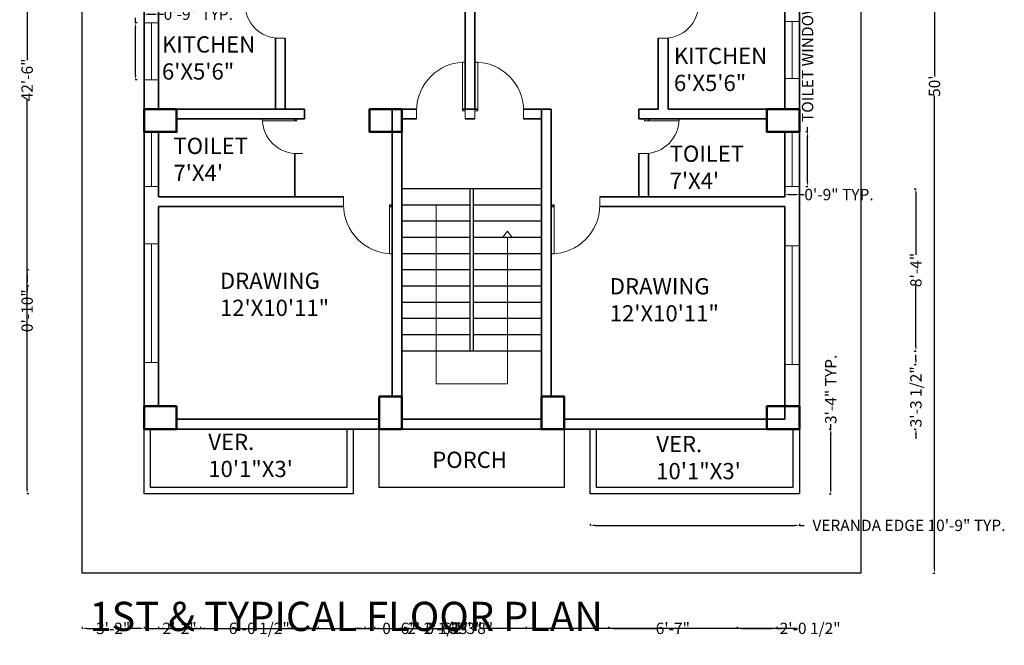
# Model space of a CAD drawing. Units: inches. Extents: x -78 to 529, y -573 to 148.
# Tile 1 of 2: x -78 to 529, y -573 to -187. Entities that reach past the tile are written whole.
import ezdxf

# ---------------------------------------------------------------- set-up
doc = ezdxf.new("R2010")
doc.units = ezdxf.units.IN
doc.header["$MEASUREMENT"] = 0
for name, color, linetype, lineweight in [('A-ANNO-DIMS', 2, 'Continuous', 18), ('A-ANNO-SYMB', 2, 'Continuous', 13), ('A-ANNO-TEXT', 7, 'Continuous', 35), ('A-AREA-IDEN', 5, 'Continuous', 18), ('A-COLS', 1, 'Continuous', 50), ('A-DOOR', 3, 'Continuous', 18), ('A-FLOR-EDGE', 7, 'Continuous', 25), ('A-FLOR-STRS', 7, 'Continuous', 25), ('A-GLAZ', 4, 'Continuous', 18), ('A-WALL', 7, 'Continuous', 35), ('C-PROP', 8, 'Continuous', 25)]:
    doc.layers.add(name, color=color, linetype=linetype, lineweight=lineweight)
doc.styles.get("Standard").update_dxf_attribs({"font": 'arial.ttf'})
doc.dimstyles.get("Standard").update_dxf_attribs({"dimtxt": 7, "dimasz": 3, "dimexe": 0.18, "dimexo": 0.0625, "dimgap": 0.09, "dimtad": 0, "dimdec": 0, "dimzin": 0, "dimdsep": 46, "dimlunit": 3, "dimtxsty": 'Standard', "dimcen": 0.09, "dimadec": 0, "dimazin": 0, "dimtfac": 1, "dimtdec": 0, "dimtofl": 0, "dimtmove": 0, "dimatfit": 3, "dimfxl": 1, "dimfxlon": 1, "dimtolj": 1, "dimtzin": 0, "dimarcsym": 0})

# ---------------------------------------------------------------- blocks, each defined once
blk = doc.blocks.new('*U2')
for p, q in [((0, 0), (0, -5)), ((30, 0), (30, -5))]:
    blk.add_line(p, q)
blk.add_lwpolyline([(0, 0), (0, 30), (1.75, 30), (1.75, 0)], close=True)
blk.add_arc((0, 0), 30, 0, 90)
blk = doc.blocks.new('*D4')
at = {"layer": 'A-ANNO-DIMS', "color": 0, "lineweight": -2, "transparency": 16777216}
for p, q in [((485.19, 71.78), (486.37, 71.78)), ((486.19, 68.78), (486.19, -222.19)), ((486.19, -525.22), (486.19, -234.25)), ((485.19, -528.22), (486.37, -528.22))]:
    blk.add_line(p, q, dxfattribs=at)
at = {"layer": 'A-ANNO-DIMS', "color": 0, "transparency": 16777216}
for points in [[(485.69, 68.78), (486.69, 68.78), (486.19, 71.78)], [(485.69, -525.22), (486.69, -525.22), (486.19, -528.22)]]:
    blk.add_solid(points, dxfattribs=at)
at = {"layer": 'Defpoints', "color": 0, "transparency": 16777216}
for p in [(440.78, 71.78), (440.78, -528.22), (486.19, -528.22)]:
    blk.add_point(p, dxfattribs=at)
at = {"layer": 'A-ANNO-DIMS', "color": 0, "transparency": 16777216, "insert": (486.19, -228.22), "char_height": 7, "attachment_point": 5, "rotation": 90}
blk.add_mtext("\\A1;50'", dxfattribs=at)
blk = doc.blocks.new('COLUMN-14X20')
blk.add_lwpolyline([(0, 20), (14, 20), (14, 0), (0, 0)], close=True)
blk = doc.blocks.new('VERANDA-EDGE')
for p, q in [((0, 0), (0, 40)), ((4, 4), (4, 40)), ((125, 40), (125, 4)), ((129, 40), (129, 0)), ((129, 0), (0, 0)), ((125, 4), (4, 4))]:
    blk.add_line(p, q)
blk = doc.blocks.new('WIN-BED-LIVING')
for p, q in [((0, 73.06), (9, 73.06)), ((4.5, 0), (4.5, 73.06)), ((0, 0), (9, 0))]:
    blk.add_line(p, q)
blk = doc.blocks.new('WIN-KITCHEN')
for p, q in [((0, 35.09), (9, 35.09)), ((4.5, 35.09), (4.5, 0)), ((0, 0), (9, 0))]:
    blk.add_line(p, q)
blk = doc.blocks.new('WIN-TOILET')
for p, q in [((4.5, 33.56), (4.5, 0)), ((0, 0), (9, 0))]:
    blk.add_line(p, q)
blk = doc.blocks.new('*D14')
at = {"layer": 'A-ANNO-DIMS', "color": 0, "lineweight": -2, "transparency": 16777216}
for p, q in [((273.91, -497.74), (273.91, -498.92)), ((276.91, -498.74), (399.91, -498.74)), ((402.91, -497.74), (402.91, -498.92)), ((402.91, -498.74), (405.91, -498.74))]:
    blk.add_line(p, q, dxfattribs=at)
at = {"layer": 'A-ANNO-DIMS', "color": 0, "transparency": 16777216}
for points in [[(276.91, -498.24), (276.91, -499.24), (273.91, -498.74)], [(399.91, -498.24), (399.91, -499.24), (402.91, -498.74)]]:
    blk.add_solid(points, dxfattribs=at)
at = {"layer": 'Defpoints', "color": 0, "transparency": 16777216}
for p in [(273.91, -479.39), (402.91, -479.39), (402.91, -498.74)]:
    blk.add_point(p, dxfattribs=at)
at = {"layer": 'A-ANNO-DIMS', "color": 0, "transparency": 16777216, "insert": (470.45, -498.74), "char_height": 7, "attachment_point": 5}
blk.add_mtext('\\A1;VERANDA EDGE 10\'-9" TYP.', dxfattribs=at)
blk = doc.blocks.new('*D15')
at = {"layer": 'A-ANNO-DIMS', "color": 0, "lineweight": -2, "transparency": 16777216}
for p, q in [((422.26, -439.39), (422.26, -436.39)), ((421.26, -439.39), (422.44, -439.39)), ((422.26, -476.39), (422.26, -442.39)), ((421.26, -479.39), (422.44, -479.39))]:
    blk.add_line(p, q, dxfattribs=at)
at = {"layer": 'A-ANNO-DIMS', "color": 0, "transparency": 16777216}
for points in [[(421.76, -442.39), (422.76, -442.39), (422.26, -439.39)], [(421.76, -476.39), (422.76, -476.39), (422.26, -479.39)]]:
    blk.add_solid(points, dxfattribs=at)
at = {"layer": 'Defpoints', "color": 0, "transparency": 16777216}
for p in [(402.91, -439.39), (422.26, -439.39), (402.91, -479.39)]:
    blk.add_point(p, dxfattribs=at)
at = {"layer": 'A-ANNO-DIMS', "color": 0, "transparency": 16777216, "insert": (422.26, -414.97), "char_height": 7, "attachment_point": 5, "rotation": 90}
blk.add_mtext('\\A1;3\'-4" TYP.', dxfattribs=at)
blk = doc.blocks.new('*D16')
at = {"layer": 'A-ANNO-DIMS', "color": 0, "lineweight": -2, "transparency": 16777216}
for p, q in [((-6.35, -189.15), (-6.35, -186.15)), ((-5.35, -189.15), (-6.53, -189.15)), ((-6.35, -221.25), (-6.35, -192.15)), ((-5.35, -224.25), (-6.53, -224.25))]:
    blk.add_line(p, q, dxfattribs=at)
at = {"layer": 'A-ANNO-DIMS', "color": 0, "transparency": 16777216}
for points in [[(-6.85, -192.15), (-5.85, -192.15), (-6.35, -189.15)], [(-6.85, -221.25), (-5.85, -221.25), (-6.35, -224.25)]]:
    blk.add_solid(points, dxfattribs=at)
at = {"layer": 'Defpoints', "color": 0, "transparency": 16777216}
for p in [(-6.35, -189.15), (-1.09, -189.15), (-1.09, -224.25)]:
    blk.add_point(p, dxfattribs=at)
at = {"layer": 'A-ANNO-DIMS', "color": 0, "transparency": 16777216, "insert": (-6.35, -116.53), "char_height": 7, "attachment_point": 5, "rotation": 90}
blk.add_mtext('\\A1;KITCHEN WINDOW 2\'-11" TYP.', dxfattribs=at)
blk = doc.blocks.new('*D17')
at = {"layer": 'A-ANNO-DIMS', "color": 0, "lineweight": -2, "transparency": 16777216}
for p, q in [((-1.09, -184.89), (-1.09, -183.71)), ((1.91, -183.89), (4.91, -183.89)), ((7.91, -184.89), (7.91, -183.71)), ((7.91, -183.89), (10.91, -183.89))]:
    blk.add_line(p, q, dxfattribs=at)
at = {"layer": 'A-ANNO-DIMS', "color": 0, "transparency": 16777216}
for points in [[(1.91, -183.39), (1.91, -184.39), (-1.09, -183.89)], [(4.91, -183.39), (4.91, -184.39), (7.91, -183.89)]]:
    blk.add_solid(points, dxfattribs=at)
at = {"layer": 'Defpoints', "color": 0, "transparency": 16777216}
for p in [(7.91, -183.89), (-1.09, -189.15), (7.91, -189.15)]:
    blk.add_point(p, dxfattribs=at)
at = {"layer": 'A-ANNO-DIMS', "color": 0, "transparency": 16777216, "insert": (32.34, -183.89), "char_height": 7, "attachment_point": 5}
blk.add_mtext('\\A1;0\'-9" TYP.', dxfattribs=at)
blk = doc.blocks.new('*D18')
at = {"layer": 'A-ANNO-DIMS', "color": 0, "lineweight": -2, "transparency": 16777216}
for p, q in [((407.95, -256.39), (407.95, -253.39)), ((406.95, -256.39), (408.13, -256.39)), ((407.95, -286.96), (407.95, -259.39)), ((406.95, -289.96), (408.13, -289.96))]:
    blk.add_line(p, q, dxfattribs=at)
at = {"layer": 'A-ANNO-DIMS', "color": 0, "transparency": 16777216}
for points in [[(407.45, -259.39), (408.45, -259.39), (407.95, -256.39)], [(407.45, -286.96), (408.45, -286.96), (407.95, -289.96)]]:
    blk.add_solid(points, dxfattribs=at)
at = {"layer": 'Defpoints', "color": 0, "transparency": 16777216}
for p in [(402.91, -256.39), (407.95, -256.39), (402.91, -289.96)]:
    blk.add_point(p, dxfattribs=at)
at = {"layer": 'A-ANNO-DIMS', "color": 0, "transparency": 16777216, "insert": (407.95, -182.44), "char_height": 7, "attachment_point": 5, "rotation": 90}
blk.add_mtext('\\A1;TOILET WINDOW 2\'-9 1/2" TYP.', dxfattribs=at)
blk = doc.blocks.new('*D19')
at = {"layer": 'A-ANNO-DIMS', "color": 0, "lineweight": -2, "transparency": 16777216}
for p, q in [((393.91, -293.99), (393.91, -295.17)), ((396.91, -294.99), (399.91, -294.99)), ((402.91, -293.99), (402.91, -295.17)), ((402.91, -294.99), (405.91, -294.99))]:
    blk.add_line(p, q, dxfattribs=at)
at = {"layer": 'A-ANNO-DIMS', "color": 0, "transparency": 16777216}
for points in [[(396.91, -294.49), (396.91, -295.49), (393.91, -294.99)], [(399.91, -294.49), (399.91, -295.49), (402.91, -294.99)]]:
    blk.add_solid(points, dxfattribs=at)
at = {"layer": 'Defpoints', "color": 0, "transparency": 16777216}
for p in [(393.91, -289.96), (402.91, -289.96), (402.91, -294.99)]:
    blk.add_point(p, dxfattribs=at)
at = {"layer": 'A-ANNO-DIMS', "color": 0, "transparency": 16777216, "insert": (427.34, -294.99), "char_height": 7, "attachment_point": 5}
blk.add_mtext('\\A1;0\'-9" TYP.', dxfattribs=at)
blk = doc.blocks.new('*D20')
at = {"layer": 'A-ANNO-DIMS', "color": 0, "lineweight": -2, "transparency": 16777216}
for p, q in [((-1.09, -561.17), (-1.09, -562.35)), ((1.91, -562.17), (188.8, -562.17)), ((399.91, -562.17), (213.02, -562.17)), ((402.91, -561.17), (402.91, -562.35))]:
    blk.add_line(p, q, dxfattribs=at)
at = {"layer": 'A-ANNO-DIMS', "color": 0, "transparency": 16777216}
for points in [[(1.91, -561.67), (1.91, -562.67), (-1.09, -562.17)], [(399.91, -561.67), (399.91, -562.67), (402.91, -562.17)]]:
    blk.add_solid(points, dxfattribs=at)
at = {"layer": 'Defpoints', "color": 0, "transparency": 16777216}
for p in [(-1.09, -479.39), (402.91, -479.39), (402.91, -562.17)]:
    blk.add_point(p, dxfattribs=at)
at = {"layer": 'A-ANNO-DIMS', "color": 0, "transparency": 16777216, "insert": (200.91, -562.17), "char_height": 7, "attachment_point": 5}
blk.add_mtext('\\A1;33\'-8"', dxfattribs=at)
blk = doc.blocks.new('*D21')
at = {"layer": 'A-ANNO-DIMS', "color": 0, "lineweight": -2, "transparency": 16777216}
for p, q in [((-72.17, 30.61), (-73.35, 30.61)), ((-73.17, 27.61), (-73.17, -212.14)), ((-73.17, -476.39), (-73.17, -236.65)), ((-72.17, -479.39), (-73.35, -479.39))]:
    blk.add_line(p, q, dxfattribs=at)
at = {"layer": 'A-ANNO-DIMS', "color": 0, "transparency": 16777216}
for points in [[(-73.67, 27.61), (-72.67, 27.61), (-73.17, 30.61)], [(-73.67, -476.39), (-72.67, -476.39), (-73.17, -479.39)]]:
    blk.add_solid(points, dxfattribs=at)
at = {"layer": 'Defpoints', "color": 0, "transparency": 16777216}
for p in [(-73.17, 30.61), (-1.09, 30.61), (-1.09, -479.39)]:
    blk.add_point(p, dxfattribs=at)
at = {"layer": 'A-ANNO-DIMS', "color": 0, "transparency": 16777216, "insert": (-73.17, -224.39), "char_height": 7, "attachment_point": 5, "rotation": 90}
blk.add_mtext('\\A1;42\'-6"', dxfattribs=at)
blk = doc.blocks.new('*D22')
at = {"layer": 'A-ANNO-DIMS', "color": 0, "lineweight": -2, "transparency": 16777216}
for p, q in [((-39.22, -561.17), (-39.22, -562.35)), ((-36.22, -562.17), (-29.54, -562.17)), ((-4.09, -562.17), (-10.76, -562.17)), ((-1.09, -561.17), (-1.09, -562.35))]:
    blk.add_line(p, q, dxfattribs=at)
at = {"layer": 'A-ANNO-DIMS', "color": 0, "transparency": 16777216}
for points in [[(-36.22, -561.67), (-36.22, -562.67), (-39.22, -562.17)], [(-4.09, -561.67), (-4.09, -562.67), (-1.09, -562.17)]]:
    blk.add_solid(points, dxfattribs=at)
at = {"layer": 'Defpoints', "color": 0, "transparency": 16777216}
for p in [(-1.09, -479.39), (-39.22, -528.22), (-1.09, -562.17)]:
    blk.add_point(p, dxfattribs=at)
at = {"layer": 'A-ANNO-DIMS', "color": 0, "transparency": 16777216, "insert": (-20.15, -562.17), "char_height": 7, "attachment_point": 5}
blk.add_mtext('\\A1;3\'-2"', dxfattribs=at)
blk = doc.blocks.new('*D24')
at = {"layer": 'A-ANNO-DIMS', "color": 0, "lineweight": -2, "transparency": 16777216}
for p, q in [((157.91, 104.73), (157.91, 105.91)), ((160.91, 105.73), (191.55, 105.73)), ((240.91, 105.73), (210.28, 105.73)), ((243.91, 104.73), (243.91, 105.91))]:
    blk.add_line(p, q, dxfattribs=at)
at = {"layer": 'A-ANNO-DIMS', "color": 0, "transparency": 16777216}
for points in [[(160.91, 106.23), (160.91, 105.23), (157.91, 105.73)], [(240.91, 106.23), (240.91, 105.23), (243.91, 105.73)]]:
    blk.add_solid(points, dxfattribs=at)
at = {"layer": 'Defpoints', "color": 0, "transparency": 16777216}
for p in [(243.91, 105.73), (157.91, -433.39), (243.91, -433.39)]:
    blk.add_point(p, dxfattribs=at)
at = {"layer": 'A-ANNO-DIMS', "color": 0, "transparency": 16777216, "insert": (200.91, 105.73), "char_height": 7, "attachment_point": 5}
blk.add_mtext('\\A1;7\'-2"', dxfattribs=at)
blk = doc.blocks.new('*D25')
at = {"layer": 'A-ANNO-DIMS', "color": 0, "lineweight": -2, "transparency": 16777216}
for p, q in [((473.73, -291.42), (474.91, -291.42)), ((474.73, -294.42), (474.73, -332.02)), ((474.73, -388.42), (474.73, -350.81)), ((473.73, -391.42), (474.91, -391.42))]:
    blk.add_line(p, q, dxfattribs=at)
at = {"layer": 'A-ANNO-DIMS', "color": 0, "transparency": 16777216}
for points in [[(474.23, -294.42), (475.23, -294.42), (474.73, -291.42)], [(474.23, -388.42), (475.23, -388.42), (474.73, -391.42)]]:
    blk.add_solid(points, dxfattribs=at)
at = {"layer": 'Defpoints', "color": 0, "transparency": 16777216}
for p in [(157.91, -291.42), (474.73, -291.42), (157.91, -391.42)]:
    blk.add_point(p, dxfattribs=at)
at = {"layer": 'A-ANNO-DIMS', "color": 0, "transparency": 16777216, "insert": (474.73, -341.42), "char_height": 7, "attachment_point": 5, "rotation": 90}
blk.add_mtext('\\A1;8\'-4"', dxfattribs=at)
blk = doc.blocks.new('*D26')
at = {"layer": 'A-ANNO-DIMS', "color": 0, "lineweight": -2, "transparency": 16777216}
for p, q in [((-72.17, -341.42), (-73.35, -341.42)), ((-73.17, -344.42), (-73.17, -348.42)), ((-72.17, -351.42), (-73.35, -351.42)), ((-73.17, -351.42), (-73.17, -354.42))]:
    blk.add_line(p, q, dxfattribs=at)
at = {"layer": 'A-ANNO-DIMS', "color": 0, "transparency": 16777216}
for points in [[(-73.67, -344.42), (-72.67, -344.42), (-73.17, -341.42)], [(-73.67, -348.42), (-72.67, -348.42), (-73.17, -351.42)]]:
    blk.add_solid(points, dxfattribs=at)
at = {"layer": 'Defpoints', "color": 0, "transparency": 16777216}
for p in [(243.91, -341.42), (-73.17, -351.42), (243.91, -351.42)]:
    blk.add_point(p, dxfattribs=at)
at = {"layer": 'A-ANNO-DIMS', "color": 0, "transparency": 16777216, "insert": (-73.17, -366.53), "char_height": 7, "attachment_point": 5, "rotation": 90}
blk.add_mtext('\\A1;0\'-10"', dxfattribs=at)
blk = doc.blocks.new('*D27')
at = {"layer": 'A-ANNO-DIMS', "color": 0, "lineweight": -2, "transparency": 16777216}
for p, q in [((166.91, -561.17), (166.91, -562.35)), ((169.91, -562.17), (172.46, -562.17)), ((193.91, -562.17), (191.36, -562.17)), ((196.91, -561.17), (196.91, -562.35))]:
    blk.add_line(p, q, dxfattribs=at)
at = {"layer": 'A-ANNO-DIMS', "color": 0, "transparency": 16777216}
for points in [[(169.91, -561.67), (169.91, -562.67), (166.91, -562.17)], [(193.91, -561.67), (193.91, -562.67), (196.91, -562.17)]]:
    blk.add_solid(points, dxfattribs=at)
at = {"layer": 'Defpoints', "color": 0, "transparency": 16777216}
for p in [(166.91, -248.39), (196.91, -248.39), (196.91, -562.17)]:
    blk.add_point(p, dxfattribs=at)
at = {"layer": 'A-ANNO-DIMS', "color": 0, "transparency": 16777216, "insert": (181.91, -562.17), "char_height": 7, "attachment_point": 5}
blk.add_mtext('\\A1;2\'-6"', dxfattribs=at)
blk = doc.blocks.new('*D29')
at = {"layer": 'A-ANNO-DIMS', "color": 0, "lineweight": -2, "transparency": 16777216}
for p, q in [((7.91, -561.17), (7.91, -562.35)), ((10.91, -562.17), (11.34, -562.17)), ((30.68, -562.17), (30.25, -562.17)), ((33.68, -561.17), (33.68, -562.35))]:
    blk.add_line(p, q, dxfattribs=at)
at = {"layer": 'A-ANNO-DIMS', "color": 0, "transparency": 16777216}
for points in [[(10.91, -561.67), (10.91, -562.67), (7.91, -562.17)], [(30.68, -561.67), (30.68, -562.67), (33.68, -562.17)]]:
    blk.add_solid(points, dxfattribs=at)
at = {"layer": 'Defpoints', "color": 0, "transparency": 16777216}
for p in [(7.91, 21.61), (33.68, 21.61), (33.68, -562.17)]:
    blk.add_point(p, dxfattribs=at)
at = {"layer": 'A-ANNO-DIMS', "color": 0, "transparency": 16777216, "insert": (20.79, -562.17), "char_height": 7, "attachment_point": 5}
blk.add_mtext('\\A1;2\'-2"', dxfattribs=at)
blk = doc.blocks.new('*D30')
at = {"layer": 'A-ANNO-DIMS', "color": 0, "lineweight": -2, "transparency": 16777216}
for p, q in [((33.68, -561.17), (33.68, -562.35)), ((36.68, -562.17), (52.37, -562.17)), ((103.2, -562.17), (87.51, -562.17)), ((106.2, -561.17), (106.2, -562.35))]:
    blk.add_line(p, q, dxfattribs=at)
at = {"layer": 'A-ANNO-DIMS', "color": 0, "transparency": 16777216}
for points in [[(36.68, -561.67), (36.68, -562.67), (33.68, -562.17)], [(103.2, -561.67), (103.2, -562.67), (106.2, -562.17)]]:
    blk.add_solid(points, dxfattribs=at)
at = {"layer": 'Defpoints', "color": 0, "transparency": 16777216}
for p in [(33.68, 21.61), (106.2, 21.61), (106.2, -562.17)]:
    blk.add_point(p, dxfattribs=at)
at = {"layer": 'A-ANNO-DIMS', "color": 0, "transparency": 16777216, "insert": (69.94, -562.17), "char_height": 7, "attachment_point": 5}
blk.add_mtext('\\A1;6\'-0 1/2"', dxfattribs=at)
blk = doc.blocks.new('*D31')
at = {"layer": 'A-ANNO-DIMS', "color": 0, "lineweight": -2, "transparency": 16777216}
for p, q in [((134.91, -561.17), (134.91, -562.35)), ((137.91, -562.17), (156.38, -562.17)), ((159.38, -561.17), (159.38, -562.35)), ((159.38, -562.17), (162.38, -562.17))]:
    blk.add_line(p, q, dxfattribs=at)
at = {"layer": 'A-ANNO-DIMS', "color": 0, "transparency": 16777216}
for points in [[(137.91, -561.67), (137.91, -562.67), (134.91, -562.17)], [(156.38, -561.67), (156.38, -562.67), (159.38, -562.17)]]:
    blk.add_solid(points, dxfattribs=at)
at = {"layer": 'Defpoints', "color": 0, "transparency": 16777216}
for p in [(134.91, 30.61), (159.38, 21.61), (159.38, -562.17)]:
    blk.add_point(p, dxfattribs=at)
at = {"layer": 'A-ANNO-DIMS', "color": 0, "transparency": 16777216, "insert": (179.99, -562.17), "char_height": 7, "attachment_point": 5}
blk.add_mtext('\\A1;2\'-0 1/2"', dxfattribs=at)
blk = doc.blocks.new('*D32')
at = {"layer": 'A-ANNO-DIMS', "color": 0, "lineweight": -2, "transparency": 16777216}
for p, q in [((159.38, -561.17), (159.38, -562.35)), ((162.38, -562.17), (187.51, -562.17)), ((231.46, -562.17), (206.34, -562.17)), ((234.46, -561.17), (234.46, -562.35))]:
    blk.add_line(p, q, dxfattribs=at)
at = {"layer": 'A-ANNO-DIMS', "color": 0, "transparency": 16777216}
for points in [[(162.38, -561.67), (162.38, -562.67), (159.38, -562.17)], [(231.46, -561.67), (231.46, -562.67), (234.46, -562.17)]]:
    blk.add_solid(points, dxfattribs=at)
at = {"layer": 'Defpoints', "color": 0, "transparency": 16777216}
for p in [(159.38, 21.61), (234.46, 21.61), (234.46, -562.17)]:
    blk.add_point(p, dxfattribs=at)
at = {"layer": 'A-ANNO-DIMS', "color": 0, "transparency": 16777216, "insert": (196.92, -562.17), "char_height": 7, "attachment_point": 5}
blk.add_mtext('\\A1;6\'-3"', dxfattribs=at)
blk = doc.blocks.new('*D33')
at = {"layer": 'A-ANNO-DIMS', "color": 0, "lineweight": -2, "transparency": 16777216}
for p, q in [((364.5, -561.17), (364.5, -562.35)), ((367.5, -562.17), (385.91, -562.17)), ((388.91, -561.17), (388.91, -562.35)), ((388.91, -562.17), (391.91, -562.17))]:
    blk.add_line(p, q, dxfattribs=at)
at = {"layer": 'A-ANNO-DIMS', "color": 0, "transparency": 16777216}
for points in [[(367.5, -561.67), (367.5, -562.67), (364.5, -562.17)], [(385.91, -561.67), (385.91, -562.67), (388.91, -562.17)]]:
    blk.add_solid(points, dxfattribs=at)
at = {"layer": 'Defpoints', "color": 0, "transparency": 16777216}
for p in [(364.5, 21.61), (388.91, 10.61), (388.91, -562.17)]:
    blk.add_point(p, dxfattribs=at)
at = {"layer": 'A-ANNO-DIMS', "color": 0, "transparency": 16777216, "insert": (409.52, -562.17), "char_height": 7, "attachment_point": 5}
blk.add_mtext('\\A1;2\'-0 1/2"', dxfattribs=at)
blk = doc.blocks.new('*D34')
at = {"layer": 'A-ANNO-DIMS', "color": 0, "lineweight": -2, "transparency": 16777216}
for p, q in [((285.28, -561.17), (285.28, -562.35)), ((288.28, -562.17), (315.48, -562.17)), ((361.5, -562.17), (334.3, -562.17)), ((364.5, -561.17), (364.5, -562.35))]:
    blk.add_line(p, q, dxfattribs=at)
at = {"layer": 'A-ANNO-DIMS', "color": 0, "transparency": 16777216}
for points in [[(288.28, -561.67), (288.28, -562.67), (285.28, -562.17)], [(361.5, -561.67), (361.5, -562.67), (364.5, -562.17)]]:
    blk.add_solid(points, dxfattribs=at)
at = {"layer": 'Defpoints', "color": 0, "transparency": 16777216}
for p in [(285.28, 21.61), (364.5, 21.61), (364.5, -562.17)]:
    blk.add_point(p, dxfattribs=at)
at = {"layer": 'A-ANNO-DIMS', "color": 0, "transparency": 16777216, "insert": (324.89, -562.17), "char_height": 7, "attachment_point": 5}
blk.add_mtext('\\A1;6\'-7"', dxfattribs=at)
blk = doc.blocks.new('*D36')
at = {"layer": 'A-ANNO-DIMS', "color": 0, "lineweight": -2, "transparency": 16777216}
for p, q in [((474.73, -396.72), (474.73, -393.72)), ((473.73, -399.72), (474.91, -399.72)), ((473.73, -439.39), (474.91, -439.39)), ((474.73, -442.39), (474.73, -445.39))]:
    blk.add_line(p, q, dxfattribs=at)
at = {"layer": 'A-ANNO-DIMS', "color": 0, "transparency": 16777216}
for points in [[(474.23, -396.72), (475.23, -396.72), (474.73, -399.72)], [(474.23, -442.39), (475.23, -442.39), (474.73, -439.39)]]:
    blk.add_solid(points, dxfattribs=at)
at = {"layer": 'Defpoints', "color": 0, "transparency": 16777216}
for p in [(402.91, -399.72), (474.73, -399.72), (402.91, -439.39)]:
    blk.add_point(p, dxfattribs=at)
at = {"layer": 'A-ANNO-DIMS', "color": 0, "transparency": 16777216, "insert": (474.73, -419.56), "char_height": 7, "attachment_point": 5, "rotation": 90}
blk.add_mtext('\\A1;3\'-3 1/2"', dxfattribs=at)
blk = doc.blocks.new('*D38')
at = {"layer": 'A-ANNO-DIMS', "color": 0, "lineweight": -2, "transparency": 16777216}
for p, q in [((131.91, -562.17), (128.91, -562.17)), ((134.91, -561.17), (134.91, -562.35)), ((140.91, -561.17), (140.91, -562.35)), ((143.91, -562.17), (146.91, -562.17))]:
    blk.add_line(p, q, dxfattribs=at)
at = {"layer": 'A-ANNO-DIMS', "color": 0, "transparency": 16777216}
for points in [[(131.91, -561.67), (131.91, -562.67), (134.91, -562.17)], [(143.91, -561.67), (143.91, -562.67), (140.91, -562.17)]]:
    blk.add_solid(points, dxfattribs=at)
at = {"layer": 'Defpoints', "color": 0, "transparency": 16777216}
for p in [(134.91, -123.39), (140.91, -123.39), (140.91, -562.17)]:
    blk.add_point(p, dxfattribs=at)
at = {"layer": 'A-ANNO-DIMS', "color": 0, "transparency": 16777216, "insert": (156.31, -562.17), "char_height": 7, "attachment_point": 5}
blk.add_mtext('\\A1;0\'-6"', dxfattribs=at)

msp = doc.modelspace()

# ---------------------------------------------------------------- linework, layer by layer
at = {"layer": 'A-ANNO-SYMB'}
for p, q in [((178.91, -301.42), (178.91, -411.47)), ((219.98, -321.42), (222.91, -317.45)), ((225.84, -321.42), (222.91, -317.45)), ((222.91, -411.47), (222.91, -321.42)), ((178.91, -411.47), (222.91, -411.47))]:
    msp.add_line(p, q, dxfattribs=at)
at = {"layer": 'A-FLOR-EDGE'}
for p, q in [((143.91, -475.39), (143.91, -439.39)), ((257.91, -439.39), (257.91, -475.39)), ((257.91, -475.39), (143.91, -475.39))]:
    msp.add_line(p, q, dxfattribs=at)
at = {"layer": 'A-FLOR-STRS'}
for p, q in [((243.91, -291.42), (157.91, -291.42)), ((199.91, -391.42), (199.91, -291.42)), ((201.91, -391.42), (201.91, -291.42)), ((199.91, -301.42), (157.91, -301.42)), ((243.91, -301.42), (201.91, -301.42)), ((199.91, -311.42), (157.91, -311.42)), ((243.91, -311.42), (201.91, -311.42)), ((199.91, -321.42), (157.91, -321.42)), ((243.91, -321.42), (201.91, -321.42)), ((199.91, -331.42), (157.91, -331.42)), ((243.91, -331.42), (201.91, -331.42)), ((199.91, -341.42), (157.91, -341.42)), ((243.91, -341.42), (201.91, -341.42)), ((199.91, -351.42), (157.91, -351.42)), ((243.91, -351.42), (201.91, -351.42)), ((199.91, -361.42), (157.91, -361.42)), ((243.91, -361.42), (201.91, -361.42)), ((199.91, -371.42), (157.91, -371.42)), ((243.91, -371.42), (201.91, -371.42)), ((199.91, -381.42), (157.91, -381.42)), ((243.91, -381.42), (201.91, -381.42)), ((243.91, -391.42), (157.91, -391.42))]:
    msp.add_line(p, q, dxfattribs=at)
at = {"layer": 'A-WALL'}
for p, q in [((-1.09, 30.61), (-1.09, -439.39)), ((402.91, 30.61), (402.91, -439.39)), ((393.91, -131.41), (393.91, -242.39)), ((196.91, -143.39), (196.91, -242.39)), ((202.91, -143.39), (202.91, -242.39)), ((7.91, -177.39), (7.91, -242.39)), ((79.91, -198.57), (79.91, -242.39)), ((85.91, -198.71), (85.91, -242.39)), ((315.91, -198.71), (315.91, -242.39)), ((321.91, -198.57), (321.91, -242.39)), ((7.91, -242.39), (97.91, -242.39)), ((97.91, -242.39), (97.91, -248.39)), ((151.91, -242.39), (151.91, -419.39)), ((151.91, -242.39), (166.93, -242.39)), ((157.91, -242.39), (157.91, -433.39)), ((195.16, -242.39), (204.66, -242.39)), ((232.89, -242.39), (249.91, -242.39)), ((243.91, -242.39), (243.91, -433.39)), ((249.91, -242.39), (249.91, -419.39)), ((303.91, -242.39), (303.91, -248.39)), ((303.91, -242.39), (315.91, -242.39)), ((321.91, -242.39), (393.91, -242.39)), ((18.91, -248.39), (97.91, -248.39)), ((91.91, -248.39), (91.91, -249.64)), ((157.91, -248.39), (166.91, -248.39)), ((196.91, -248.39), (202.91, -248.39)), ((232.91, -248.39), (243.91, -248.39)), ((303.91, -248.39), (382.91, -248.39)), ((309.91, -248.39), (309.91, -249.64)), ((7.91, -256.39), (7.91, -296.39)), ((393.91, -256.39), (393.91, -296.39)), ((91.91, -269.68), (91.91, -296.39)), ((303.91, -269.71), (303.91, -296.39)), ((309.91, -269.57), (309.91, -296.39)), ((7.91, -296.39), (121.91, -296.39)), ((279.91, -296.39), (393.91, -296.39)), ((7.91, -302.39), (121.93, -302.39)), ((7.91, -302.39), (7.91, -425.39)), ((150.16, -302.39), (151.91, -302.39)), ((249.91, -302.39), (251.66, -302.39)), ((279.89, -302.39), (393.91, -302.39)), ((393.91, -302.39), (393.91, -433.39)), ((18.91, -433.39), (143.91, -433.39)), ((157.91, -433.39), (243.91, -433.39)), ((257.91, -433.39), (393.91, -433.39)), ((-1.09, -439.39), (402.91, -439.39))]:
    msp.add_line(p, q, dxfattribs=at)
at = {"layer": 'C-PROP'}
msp.add_lwpolyline([(-39.22, 71.78), (440.78, 71.78), (440.78, -528.22), (-39.22, -528.22)], close=True, dxfattribs=at)

# ---------------------------------------------------------------- block references
at = {"layer": 'A-COLS'}
for p, rotation in [((-1.09, -242.39), 270), ((137.91, -242.39), 270.0000000000003), ((382.91, -242.39), 269.9999999999999), ((-1.09, -425.39), 270), ((382.91, -425.39), 270.0000000000001)]:
    msp.add_blockref('COLUMN-14X20', p, dxfattribs=dict(at, rotation=rotation))
for p in [(143.91, -439.39), (243.91, -439.39)]:
    msp.add_blockref('COLUMN-14X20', p, dxfattribs=at)
at = {"layer": 'A-DOOR', "yscale": 0.710672036818973, "zscale": 0.710672036818973}
for p, xscale, rotation in [((82.36, -177.39), -0.710672036818973, 90), ((319.46, -177.39), 0.710672036818973, 270), ((93.16, -248.39), -0.710672036818973, 90), ((307.46, -248.39), 0.710672036818973, 270)]:
    msp.add_blockref('*U2', p, dxfattribs=dict(at, xscale=xscale, rotation=rotation))
at = {"layer": 'A-DOOR', "xscale": -1}
msp.add_blockref('*U2', (196.91, -243.39), dxfattribs=at)
at = {"layer": 'A-DOOR'}
msp.add_blockref('*U2', (202.91, -243.39), dxfattribs=at)
at = {"layer": 'A-DOOR', "rotation": 180}
msp.add_blockref('*U2', (151.91, -301.39), dxfattribs=at)
at = {"layer": 'A-DOOR', "xscale": -1, "rotation": 180}
msp.add_blockref('*U2', (249.91, -301.39), dxfattribs=at)
at = {"layer": 'A-FLOR-EDGE'}
for p in [(-1.09, -479.39), (273.91, -479.39)]:
    msp.add_blockref('VERANDA-EDGE', p, dxfattribs=at)
at = {"layer": 'A-GLAZ'}
for name, p in [('WIN-KITCHEN', (-1.09, -224.25)), ('WIN-TOILET', (-1.09, -289.96)), ('WIN-TOILET', (393.91, -289.96)), ('WIN-BED-LIVING', (-1.09, -398.34)), ('WIN-BED-LIVING', (393.91, -399.72))]:
    msp.add_blockref(name, p, dxfattribs=at)
at = {"layer": 'A-GLAZ', "rotation": 180}
msp.add_blockref('WIN-KITCHEN', (402.91, -188.35), dxfattribs=at)

# ---------------------------------------------------------------- texts
at = {"layer": 'A-ANNO-TEXT', "insert": (-34.78, -545.81), "char_height": 18, "attachment_point": 1}
msp.add_mtext_dynamic_manual_height_columns('1ST & TYPICAL FLOOR PLAN', width=415.3064, gutter_width=1, heights=[0], dxfattribs=at)
at = {"layer": 'A-AREA-IDEN', "char_height": 10, "attachment_point": 1}
for s, insert in [('KITCHEN\\P6\'X5\'6"', (9.93, -197.5)), ('KITCHEN\\P6\'X5\'6"', (325.56, -204.56)), ("TOILET\\P7'X4'", (17.03, -259.99)), ("TOILET\\P7'X4'", (322.91, -264.82)), ('DRAWING\\P12\'X10\'11"', (45.69, -343.08)), ('DRAWING\\P12\'X10\'11"', (286, -346.47)), ('VER.\\P10\'1"X3\'', (38.5, -442.32)), ('VER.\\P10\'1"X3\'', (314.64, -443.65)), ('PORCH', (176.57, -453.36))]:
    msp.add_mtext_dynamic_manual_height_columns(s, width=71.5571, gutter_width=1, heights=[0], dxfattribs=dict(at, insert=insert))

# ---------------------------------------------------------------- dimensions: what is measured, and where the dimension line sits
at = {"layer": 'A-ANNO-DIMS'}
for base, p1, p2, picture, middle in [((243.91, 105.73), (157.91, -433.39), (243.91, -433.39), '*D24', (200.91, 105.73)), ((159.38, -562.17), (134.91, 30.61), (159.38, 21.61), '*D31', (179.99, -562.17)), ((33.68, -562.17), (7.91, 21.61), (33.68, 21.61), '*D29', (20.79, -562.17)), ((106.2, -562.17), (33.68, 21.61), (106.2, 21.61), '*D30', (69.94, -562.17)), ((234.46, -562.17), (159.38, 21.61), (234.46, 21.61), '*D32', (196.92, -562.17)), ((364.5, -562.17), (285.28, 21.61), (364.5, 21.61), '*D34', (324.89, -562.17)), ((388.91, -562.17), (364.5, 21.61), (388.91, 10.61), '*D33', (409.52, -562.17)), ((140.91, -562.17), (134.91, -123.39), (140.91, -123.39), '*D38', (156.31, -562.17)), ((196.91, -562.17), (166.91, -248.39), (196.91, -248.39), '*D27', (181.91, -562.17)), ((-1.09, -562.17), (-39.22, -528.22), (-1.09, -479.39), '*D22', (-20.15, -562.17)), ((402.91, -562.17), (-1.09, -479.39), (402.91, -479.39), '*D20', (200.91, -562.17))]:
    dim = msp.add_linear_dim(base=base, p1=p1, p2=p2, dimstyle='Standard', override={"dimdec": 1, "dimlfac": 1, "dimrnd": 0, "dimzin": 1, "dimdsep": 46, "dimlunit": 4, "dimfrac": 2}, dxfattribs=at)
    dim.commit()
    dim.dimension.update_dxf_attribs({"geometry": picture, "text_midpoint": middle})
for base, p1, p2, override, picture, middle in [((486.19, -528.22), (440.78, 71.78), (440.78, -528.22), {"dimclrd": 0, "dimclre": 0, "dimclrt": 0}, '*D4', (486.19, -228.22)), ((-73.17, 30.61), (-1.09, -479.39), (-1.09, 30.61), {"dimdec": 1, "dimlfac": 1, "dimrnd": 0, "dimzin": 1, "dimdsep": 46, "dimlunit": 4, "dimfrac": 2}, '*D21', (-73.17, -224.39)), ((474.73, -291.42), (157.91, -391.42), (157.91, -291.42), {"dimdec": 1, "dimlfac": 1, "dimrnd": 0, "dimzin": 1, "dimdsep": 46, "dimlunit": 4, "dimfrac": 2}, '*D25', (474.73, -341.42)), ((-73.17, -351.42), (243.91, -341.42), (243.91, -351.42), {"dimdec": 1, "dimlfac": 1, "dimrnd": 0, "dimzin": 1, "dimdsep": 46, "dimlunit": 4, "dimfrac": 2}, '*D26', (-73.17, -366.53)), ((474.73, -399.72), (402.91, -439.39), (402.91, -399.72), {"dimdec": 1, "dimlfac": 1, "dimrnd": 0, "dimzin": 1, "dimdsep": 46, "dimlunit": 4, "dimfrac": 2}, '*D36', (474.73, -419.56))]:
    dim = msp.add_linear_dim(base=base, p1=p1, p2=p2, angle=90, dimstyle='Standard', override=override, dxfattribs=at)
    dim.commit()
    dim.dimension.update_dxf_attribs({"geometry": picture, "text_midpoint": middle})
for base, p1, p2, text, picture, middle in [((-6.35, -189.15), (-1.09, -224.25), (-1.09, -189.15), 'KITCHEN WINDOW <> TYP.', '*D16', (-6.35, -116.53)), ((407.95, -256.39), (402.91, -289.96), (402.91, -256.39), 'TOILET WINDOW <> TYP.', '*D18', (407.95, -182.44)), ((422.26, -439.39), (402.91, -479.39), (402.91, -439.39), '<> TYP.', '*D15', (422.26, -414.97))]:
    dim = msp.add_linear_dim(base=base, p1=p1, p2=p2, angle=90, text=text, dimstyle='Standard', override={"dimdec": 1, "dimlfac": 1, "dimrnd": 0, "dimzin": 1, "dimdsep": 46, "dimlunit": 4, "dimfrac": 2}, dxfattribs=at)
    dim.commit()
    dim.dimension.update_dxf_attribs({"geometry": picture, "text_midpoint": middle})
for base, p1, p2, text, picture, middle in [((7.91, -183.89), (-1.09, -189.15), (7.91, -189.15), '<> TYP.', '*D17', (32.34, -183.89)), ((402.91, -294.99), (393.91, -289.96), (402.91, -289.96), '<> TYP.', '*D19', (427.34, -294.99)), ((402.91, -498.74), (273.91, -479.39), (402.91, -479.39), 'VERANDA EDGE <> TYP.', '*D14', (470.45, -498.74))]:
    dim = msp.add_linear_dim(base=base, p1=p1, p2=p2, text=text, dimstyle='Standard', override={"dimdec": 1, "dimlfac": 1, "dimrnd": 0, "dimzin": 1, "dimdsep": 46, "dimlunit": 4, "dimfrac": 2}, dxfattribs=at)
    dim.commit()
    dim.dimension.update_dxf_attribs({"geometry": picture, "text_midpoint": middle})

doc.saveas('drawing.dxf')
